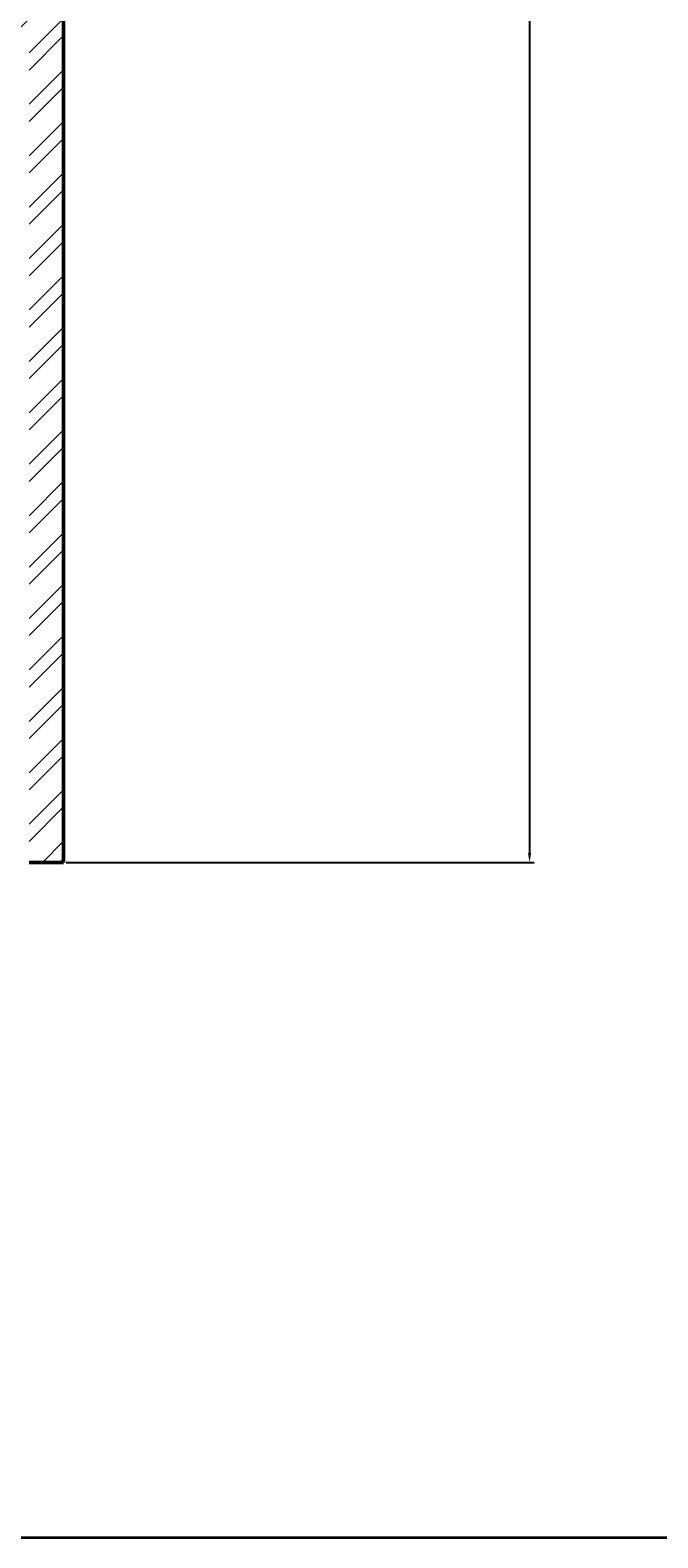
# Model space of a CAD drawing. Units: inches. Extents: x -31485 to -28799, y 18003 to 19130.
# Tile 3 of 15: x -30670 to -30506, y 18003 to 18398. Entities that reach past the tile are written whole.
import ezdxf

# ---------------------------------------------------------------- set-up
doc = ezdxf.new("R2010")
doc.units = ezdxf.units.IN
for name, color, linetype, lineweight in [('A-ANNO-DIMS', 2, 'Continuous', 18), ('A-ANNO-TTLB', 7, 'Continuous', 35), ('A-WALL', 7, 'Continuous', 50), ('A-WALL-PATT', 8, 'Continuous', 13)]:
    doc.layers.add(name, color=color, linetype=linetype, lineweight=lineweight)
doc.styles.get("Standard").update_dxf_attribs({"font": 'arial.ttf'})
doc.dimstyles.new('ISO-25', dxfattribs={"dimtxt": 2.5, "dimasz": 2.5, "dimexe": 1.25, "dimexo": 0.625, "dimtad": 1, "dimdec": 0, "dimlunit": 3, "dimtxsty": 'Standard', "dimcen": 2.5, "dimadec": 0, "dimazin": 0, "dimtfac": 1, "dimtdec": 0, "dimtmove": 0, "dimatfit": 3, "dimfxl": 1, "dimarcsym": 0})

# ---------------------------------------------------------------- blocks, each defined once
blk = doc.blocks.new('*D199')
at = {"layer": 'A-ANNO-DIMS', "color": 0, "lineweight": -2, "transparency": 16777216}
for p, q in [((-30660.9, 18823.8), (-30538.22, 18823.8)), ((-30539.47, 18821.3), (-30539.47, 18182.3)), ((-30660.9, 18179.8), (-30538.22, 18179.8))]:
    blk.add_line(p, q, dxfattribs=at)
at = {"layer": 'A-ANNO-DIMS', "color": 0, "transparency": 16777216}
for points in [[(-30539.88, 18821.3), (-30539.05, 18821.3), (-30539.47, 18823.8)], [(-30539.88, 18182.3), (-30539.05, 18182.3), (-30539.47, 18179.8)]]:
    blk.add_solid(points, dxfattribs=at)
at = {"layer": 'Defpoints', "color": 0, "transparency": 16777216}
for p in [(-30661.53, 18823.8), (-30661.53, 18179.8), (-30539.47, 18179.8)]:
    blk.add_point(p, dxfattribs=at)
at = {"layer": 'A-ANNO-DIMS', "color": 0, "transparency": 16777216, "insert": (-30548.27, 18501.8), "char_height": 2.5, "attachment_point": 5, "rotation": 90}
blk.add_mtext('{\\H6.4x;53\'-8"}', dxfattribs=at)

msp = doc.modelspace()

# ---------------------------------------------------------------- hatches: boundary and pattern name
at = {"layer": 'A-WALL-PATT'}
h = msp.add_hatch(dxfattribs=at)
h.set_pattern_fill('ANSI32', color=256)
h.set_pattern_definition([(45, (-1687.357, -0.313), (-6.735192, 6.735192), []), (45, (-1682.867, -0.313), (-6.735192, 6.735192), [])])
h.paths.add_polyline_path([(-31156.53, 18823.8), (-31209.53, 18823.8), (-31209.53, 18761.8), (-31200.53, 18761.8), (-31200.53, 18814.8), (-31156.53, 18814.8)], flags=17)
h.paths.add_polyline_path([(-31022.53, 18823.8), (-31118.53, 18823.8), (-31118.53, 18814.8), (-31074.53, 18814.8), (-31074.53, 18720.79), (-31070.96, 18720.79), (-31068.53, 18720.76), (-31068.53, 18814.8), (-31022.53, 18814.8)], flags=17)
h.paths.add_polyline_path([(-30754.53, 18823.8), (-30850.53, 18823.8), (-30850.53, 18814.8), (-30806.53, 18814.8), (-30806.53, 18723.1), (-30800.53, 18723.1), (-30800.53, 18814.8), (-30754.53, 18814.8)], flags=17)
h.paths.add_polyline_path([(-30661.53, 18823.8), (-30716.53, 18823.8), (-30716.53, 18814.8), (-30670.53, 18814.8), (-30670.53, 18761.8), (-30661.53, 18761.8)], flags=17)
h.paths.add_polyline_path([(-30986.92, 18670.8), (-31068.53, 18670.8), (-31068.53, 18684.76), (-31074.53, 18684.76), (-31074.53, 18670.8), (-31200.53, 18670.8), (-31200.53, 18723.8), (-31209.53, 18723.8), (-31209.53, 18641.8), (-31200.53, 18641.8), (-31200.53, 18664.8), (-31104.53, 18664.8), (-31104.53, 18628.93), (-31098.53, 18628.93), (-31098.53, 18664.8), (-30986.92, 18664.8)], flags=17)
h.paths.add_polyline_path([(-30661.53, 18723.8), (-30670.53, 18723.8), (-30670.53, 18670.8), (-30800.53, 18670.8), (-30800.53, 18687.1), (-30806.53, 18687.1), (-30806.53, 18670.8), (-30885.6, 18670.8), (-30885.6, 18667.8), (-30885.6, 18664.8), (-30760.53, 18664.8), (-30760.53, 18625.8), (-30754.53, 18625.8), (-30754.53, 18664.8), (-30670.53, 18664.8), (-30670.53, 18641.8), (-30661.53, 18641.8)], flags=17)
h.paths.add_polyline_path([(-31200.53, 18574.8), (-31188.56, 18574.8), (-31188.56, 18580.8), (-31200.53, 18580.8), (-31200.53, 18603.8), (-31209.53, 18603.8), (-31209.53, 18557.8), (-31200.53, 18557.8)], flags=17)
h.paths.add_polyline_path([(-31098.53, 18592.93), (-31104.53, 18592.93), (-31104.53, 18580.8), (-31164.56, 18580.8), (-31164.56, 18574.8), (-31104.53, 18574.8), (-31104.53, 18514.8), (-31200.53, 18514.8), (-31200.53, 18531.8), (-31209.53, 18531.8), (-31209.53, 18473.8), (-31200.53, 18473.8), (-31200.53, 18508.8), (-31056.53, 18508.8), (-31056.53, 18501.62), (-31050.53, 18501.62), (-31050.53, 18514.8), (-31098.53, 18514.8)], flags=17)
h.paths.add_polyline_path([(-30661.53, 18531.8), (-30670.53, 18531.8), (-30670.53, 18514.8), (-30754.53, 18514.8), (-30754.53, 18574.8), (-30700.75, 18574.8), (-30700.75, 18577.44), (-30700.75, 18580.8), (-30754.53, 18580.8), (-30754.53, 18589.8), (-30760.53, 18589.8), (-30760.53, 18514.8), (-30820.53, 18514.8), (-30820.53, 18499.26), (-30814.53, 18499.26), (-30814.53, 18508.8), (-30670.53, 18508.8), (-30670.53, 18473.8), (-30661.53, 18473.8)], flags=17)
h.paths.add_polyline_path([(-30661.53, 18435.8), (-30670.53, 18435.8), (-30670.53, 18400.8), (-30814.53, 18400.8), (-30814.53, 18413.15), (-30820.53, 18413.15), (-30820.53, 18400.8), (-30932.53, 18400.8), (-30932.53, 18664.8), (-30921.6, 18664.8), (-30921.6, 18670.8), (-30932.53, 18670.8), (-30932.53, 18814.8), (-30888.53, 18814.8), (-30888.53, 18823.8), (-30984.53, 18823.8), (-30984.53, 18814.8), (-30938.53, 18814.8), (-30938.53, 18670.8), (-30950.92, 18670.8), (-30950.92, 18664.8), (-30938.53, 18664.8), (-30938.53, 18400.8), (-31050.53, 18400.8), (-31050.53, 18411.18), (-31056.53, 18411.18), (-31056.53, 18400.8), (-31200.53, 18400.8), (-31200.53, 18435.8), (-31209.53, 18435.8), (-31209.53, 18179.8), (-31200.53, 18179.8), (-31200.53, 18394.8), (-31001.53, 18394.8), (-31001.53, 18179.8), (-30954.53, 18179.8), (-30954.53, 18188.8), (-30995.53, 18188.8), (-30995.53, 18394.8), (-30875.53, 18394.8), (-30875.53, 18188.8), (-30916.53, 18188.8), (-30916.53, 18179.8), (-30869.53, 18179.8), (-30869.53, 18394.8), (-30670.53, 18394.8), (-30670.53, 18179.8), (-30661.53, 18179.8)])

# ---------------------------------------------------------------- linework, layer by layer
at = {"layer": 'A-ANNO-TTLB'}
msp.add_lwpolyline([(-31485.1, 19129.94), (-28798.64, 19129.94), (-28798.64, 18002.86), (-31485.1, 18002.86)], close=True, dxfattribs=at)
at = {"layer": 'A-WALL'}
for p, q in [((-30661.53, 18823.8), (-30661.53, 18179.8)), ((-30661.53, 18179.8), (-30670.53, 18179.8))]:
    msp.add_line(p, q, dxfattribs=at)

# ---------------------------------------------------------------- dimensions: what is measured, and where the dimension line sits
at = {"layer": 'A-ANNO-DIMS'}
dim = msp.add_linear_dim(base=(-30539.47, 18179.8), p1=(-30661.53, 18823.8), p2=(-30661.53, 18179.8), angle=90, text='{\\H6.4x;<>}', dimstyle='ISO-25', override={"dimclrd": 0, "dimclre": 0, "dimclrt": 0}, dxfattribs=at)
dim.commit()
dim.dimension.update_dxf_attribs({"geometry": '*D199', "text_midpoint": (-30548.27, 18501.8)})

doc.saveas('drawing.dxf')
